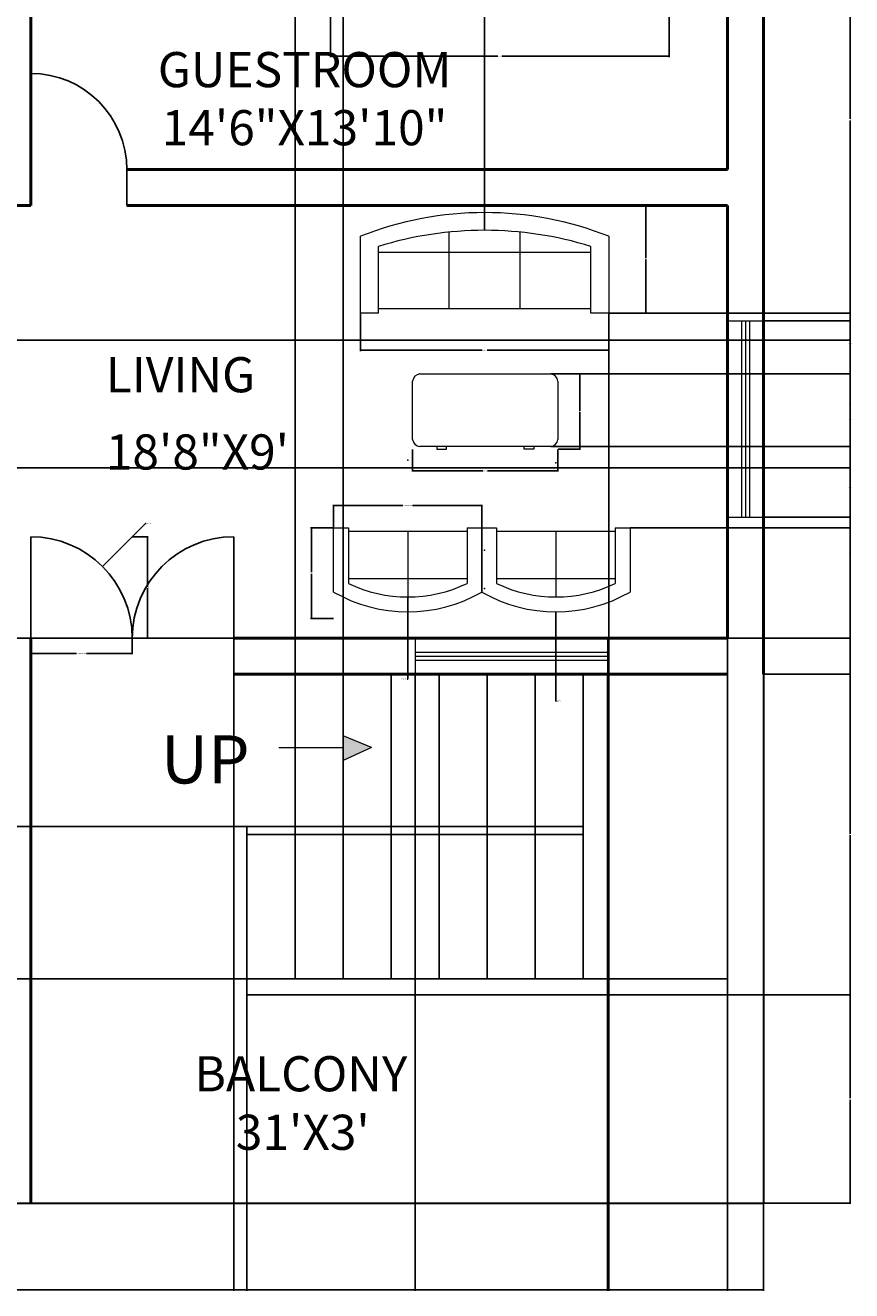
# Model space of a CAD drawing. Units: feet. Extents: x 2387 to 2818, y 1569 to 2046.
# Tile 3 of 4: x 2611 to 2818, y 1569 to 1885. Entities that reach past the tile are written whole.
import ezdxf

# ---------------------------------------------------------------- set-up
doc = ezdxf.new("R2010")
doc.units = ezdxf.units.FT
for name, color, linetype, lineweight in [('A-ANNO-DIMS', 2, 'Continuous', 18), ('A-ANNO-SYMB', 7, 'Continuous', 18), ('A-ANNO-TEXT', 7, 'Continuous', 18), ('A-AREA-IDEN', 7, 'Continuous', 18), ('A-DOOR', 3, 'Continuous', 25), ('A-FLOR-BALC', 7, 'Continuous', 30), ('A-FLOR-STRS', 7, 'Continuous', 25), ('A-FURN', 8, 'Continuous', 18), ('A-GLAZ', 4, 'Continuous', 18), ('A-WALL', 7, 'Continuous', 50)]:
    doc.layers.add(name, color=color, linetype=linetype, lineweight=lineweight)
doc.styles.get("Standard").update_dxf_attribs({"font": 'arial.ttf'})
doc.dimstyles.get("Standard").update_dxf_attribs({"dimtxt": 0.18, "dimasz": 0.18, "dimexe": 0.18, "dimexo": 0.0625, "dimgap": 0.09, "dimtad": 0, "dimtih": 1, "dimtoh": 1, "dimdec": 4, "dimzin": 0, "dimdsep": 46, "dimtxsty": 'Standard', "dimcen": 0.09, "dimadec": 0, "dimazin": 0, "dimtfac": 1, "dimtdec": 4, "dimtofl": 0, "dimtmove": 0, "dimatfit": 3, "dimfxl": 1, "dimtolj": 1, "dimtzin": 0, "dimarcsym": 0})

# ---------------------------------------------------------------- blocks, each defined once
blk = doc.blocks.new('Sofa - Roundback 7 ft.')
for p, q in [((-12.00002, -32.4421), (-12.00003, -6.5971)), ((11.99997, -32.4421), (11.99998, -6.5971)), ((-36.000027, -34), (-36.000027, -11.4696)), ((35.99998, -34), (35.99998, -11.4696)), ((-35.999844, -13.3819), (35.9998, -13.3819)), ((-36.000027, -32.4421), (35.99998, -32.4421))]:
    blk.add_line(p, q)
for points in [[(-36.000027, -34), (-42.000027, -34), (-42.000027, -8)], [(41.99998, -8), (41.99998, -34), (35.99998, -34)]]:
    blk.add_lwpolyline(points)
for centre, radius, start, end in [((0, -114.25), 114.25, 68.43141, 111.5686), ((-0.00001, -127.1968), 121.1968, 72.72033, 107.2797)]:
    blk.add_arc(centre, radius, start, end)
blk = doc.blocks.new('Desk - 30 x 60 in.')
for p, q in [((-26.999995, 0), (26.999995, 0)), ((-29.999995, -27), (-29.999995, -3)), ((29.999995, -3), (29.999995, -27)), ((26.999995, -30), (-26.999995, -30)), ((-20.000005, -30), (-20.000005, -31)), ((-20.000005, -31), (-16.000005, -31)), ((-16.000005, -31), (-16.000005, -30)), ((15.999995, -31), (15.999995, -30)), ((19.999995, -31), (15.999995, -31)), ((19.999995, -30), (19.999995, -31))]:
    blk.add_line(p, q)
for centre, start, end in [((-26.499995, -3.5), 98.1301, 171.8699), ((26.499995, -3.5), 8.130102, 81.8699), ((-26.499995, -26.5), 188.1301, 261.8699), ((26.499995, -26.5), 278.1301, 351.8699)]:
    blk.add_arc(centre, 3.535534, start, end)
blk = doc.blocks.new('Sofa - Roundback Loveseat 5 ft.')
for p, q in [((0, -32.44198), (0, -5.99998)), ((-24, -33.99998), (-24, -11.46958)), ((-23.9998, -13.38178), (23.99986, -13.38178)), ((24.00004, -33.99998), (24.00004, -11.46958)), ((-24, -32.44198), (24.00004, -32.44198))]:
    blk.add_line(p, q)
for points in [[(-24, -33.99998), (-30, -33.99998), (-30, -7.99998)], [(30.00004, -7.99998), (30.00004, -33.99998), (24.00004, -33.99998)]]:
    blk.add_lwpolyline(points)
for centre, radius, start, end in [((0, -60.24998), 60.24998, 60.13715, 119.8628), ((0, -61.38438), 55.38444, 64.32083, 115.6792)]:
    blk.add_arc(centre, radius, start, end)
blk = doc.blocks.new('DOOR-PAIRED-LEAF')
blk.add_line((0, 0), (0, 25.34))
blk.add_arc((0, 0), 25.34, 0, 90)
blk = doc.blocks.new('DOOR-BEDROOM-SWING')
blk.add_line((0, 9), (0, 0))
blk.add_arc((24, 9), 24, 90, 180)
blk = doc.blocks.new('*D12')
at = {"layer": 'A-ANNO-DIMS', "color": 0, "lineweight": -2, "transparency": 16777216}
for p, q in [((2687.62, 1893.93), (2687.62, 1876.9)), ((2772.16, 1893.93), (2772.16, 1876.9)), ((2687.8, 1877.08), (2729.36, 1877.08)), ((2771.98, 1877.08), (2730.42, 1877.08))]:
    blk.add_line(p, q, dxfattribs=at)
at = {"layer": 'A-ANNO-DIMS', "color": 0, "transparency": 16777216}
for points in [[(2687.8, 1877.11), (2687.8, 1877.05), (2687.62, 1877.08)], [(2771.98, 1877.11), (2771.98, 1877.05), (2772.16, 1877.08)]]:
    blk.add_solid(points, dxfattribs=at)
at = {"layer": 'Defpoints', "color": 0, "transparency": 16777216}
for p in [(2687.62, 1893.99), (2772.16, 1893.99), (2772.16, 1877.08)]:
    blk.add_point(p, dxfattribs=at)
at = {"layer": 'A-ANNO-DIMS', "color": 0, "transparency": 16777216, "insert": (2729.89, 1877.08), "char_height": 0.18, "attachment_point": 5}
blk.add_mtext('\\A1;85 TYP.', dxfattribs=at)
blk = doc.blocks.new('*D13')
at = {"layer": 'A-ANNO-DIMS', "color": 0, "lineweight": -2, "transparency": 16777216}
for p, q in [((2688.38, 1759.47), (2688.38, 1765.14)), ((2688.56, 1764.96), (2705.67, 1764.96)), ((2725.22, 1764.96), (2708.11, 1764.96)), ((2725.4, 1759.47), (2725.4, 1765.14))]:
    blk.add_line(p, q, dxfattribs=at)
at = {"layer": 'A-ANNO-DIMS', "color": 0, "transparency": 16777216}
for points in [[(2688.56, 1764.99), (2688.56, 1764.93), (2688.38, 1764.96)], [(2725.22, 1764.99), (2725.22, 1764.93), (2725.4, 1764.96)]]:
    blk.add_solid(points, dxfattribs=at)
at = {"layer": 'Defpoints', "color": 0, "transparency": 16777216}
for p in [(2688.38, 1764.96), (2688.38, 1759.41), (2725.4, 1759.41)]:
    blk.add_point(p, dxfattribs=at)
at = {"layer": 'A-ANNO-DIMS', "color": 0, "transparency": 16777216, "insert": (2706.89, 1764.96), "char_height": 0.18, "attachment_point": 5}
blk.add_mtext('\\A1;LOVESEAT 37 TYP.', dxfattribs=at)
blk = doc.blocks.new('*D14')
at = {"layer": 'A-ANNO-DIMS', "color": 0, "lineweight": -2, "transparency": 16777216}
for p, q in [((2688.31, 1759.41), (2682.64, 1759.41)), ((2682.82, 1759.23), (2682.82, 1748.28)), ((2682.82, 1736.96), (2682.82, 1747.91)), ((2688.31, 1736.78), (2682.64, 1736.78))]:
    blk.add_line(p, q, dxfattribs=at)
at = {"layer": 'A-ANNO-DIMS', "color": 0, "transparency": 16777216}
for points in [[(2682.79, 1759.23), (2682.85, 1759.23), (2682.82, 1759.41)], [(2682.79, 1736.96), (2682.85, 1736.96), (2682.82, 1736.78)]]:
    blk.add_solid(points, dxfattribs=at)
at = {"layer": 'Defpoints', "color": 0, "transparency": 16777216}
for p in [(2688.38, 1759.41), (2682.82, 1736.78), (2688.38, 1736.78)]:
    blk.add_point(p, dxfattribs=at)
at = {"layer": 'A-ANNO-DIMS', "color": 0, "transparency": 16777216, "insert": (2682.82, 1748.09), "char_height": 0.18, "attachment_point": 5}
blk.add_mtext('\\A1;23 TYP.', dxfattribs=at)
blk = doc.blocks.new('*D15')
at = {"layer": 'A-ANNO-DIMS', "color": 0, "lineweight": -2, "transparency": 16777216}
for p, q in [((2612.74, 1731.76), (2612.74, 1727.84)), ((2638.08, 1731.76), (2638.08, 1727.84)), ((2612.92, 1728.02), (2624.12, 1728.02)), ((2637.9, 1728.02), (2626.69, 1728.02))]:
    blk.add_line(p, q, dxfattribs=at)
at = {"layer": 'A-ANNO-DIMS', "color": 0, "transparency": 16777216}
for points in [[(2612.92, 1728.05), (2612.92, 1727.99), (2612.74, 1728.02)], [(2637.9, 1728.05), (2637.9, 1727.99), (2638.08, 1728.02)]]:
    blk.add_solid(points, dxfattribs=at)
at = {"layer": 'Defpoints', "color": 0, "transparency": 16777216}
for p in [(2612.74, 1731.82), (2638.08, 1731.82), (2638.08, 1728.02)]:
    blk.add_point(p, dxfattribs=at)
at = {"layer": 'A-ANNO-DIMS', "color": 0, "transparency": 16777216, "insert": (2625.41, 1728.02), "char_height": 0.18, "attachment_point": 5}
blk.add_mtext('\\A1;DOOR LEAF 25 TYP.', dxfattribs=at)
blk = doc.blocks.new('*D16')
at = {"layer": 'A-ANNO-DIMS', "color": 0, "lineweight": -2, "transparency": 16777216}
for p, q in [((2638.14, 1757.17), (2642.06, 1757.17)), ((2641.88, 1756.99), (2641.88, 1744.68)), ((2641.88, 1732), (2641.88, 1744.31)), ((2638.14, 1731.82), (2642.06, 1731.82))]:
    blk.add_line(p, q, dxfattribs=at)
at = {"layer": 'A-ANNO-DIMS', "color": 0, "transparency": 16777216}
for points in [[(2641.85, 1756.99), (2641.91, 1756.99), (2641.88, 1757.17)], [(2641.85, 1732), (2641.91, 1732), (2641.88, 1731.82)]]:
    blk.add_solid(points, dxfattribs=at)
at = {"layer": 'Defpoints', "color": 0, "transparency": 16777216}
for p in [(2638.08, 1757.17), (2641.88, 1757.17), (2638.08, 1731.82)]:
    blk.add_point(p, dxfattribs=at)
at = {"layer": 'A-ANNO-DIMS', "color": 0, "transparency": 16777216, "insert": (2641.88, 1744.5), "char_height": 0.18, "attachment_point": 5}
blk.add_mtext('\\A1;25 TYP.', dxfattribs=at)
blk = doc.blocks.new('*D21')
at = {"layer": 'A-ANNO-DIMS', "color": 0, "lineweight": -2, "transparency": 16777216}
for p, q in [((2695.12, 1812.93), (2695.12, 1803.52)), ((2757.09, 1812.93), (2757.09, 1803.52)), ((2695.3, 1803.7), (2725.51, 1803.7)), ((2756.91, 1803.7), (2726.7, 1803.7))]:
    blk.add_line(p, q, dxfattribs=at)
at = {"layer": 'A-ANNO-DIMS', "color": 0, "transparency": 16777216}
for points in [[(2695.3, 1803.73), (2695.3, 1803.67), (2695.12, 1803.7)], [(2756.91, 1803.73), (2756.91, 1803.67), (2757.09, 1803.7)]]:
    blk.add_solid(points, dxfattribs=at)
at = {"layer": 'Defpoints', "color": 0, "transparency": 16777216}
for p in [(2695.12, 1812.99), (2757.09, 1812.99), (2757.09, 1803.7)]:
    blk.add_point(p, dxfattribs=at)
at = {"layer": 'A-ANNO-DIMS', "color": 0, "transparency": 16777216, "insert": (2726.1, 1803.7), "char_height": 0.18, "attachment_point": 5}
blk.add_mtext('\\A1;SOFA 62', dxfattribs=at)
blk = doc.blocks.new('*D22')
at = {"layer": 'A-ANNO-DIMS', "color": 0, "lineweight": -2, "transparency": 16777216}
for p, q in [((2757.15, 1840.04), (2766.56, 1840.04)), ((2766.38, 1839.86), (2766.38, 1826.7)), ((2766.38, 1813.17), (2766.38, 1826.34)), ((2757.15, 1812.99), (2766.56, 1812.99))]:
    blk.add_line(p, q, dxfattribs=at)
at = {"layer": 'A-ANNO-DIMS', "color": 0, "transparency": 16777216}
for points in [[(2766.35, 1839.86), (2766.41, 1839.86), (2766.38, 1840.04)], [(2766.35, 1813.17), (2766.41, 1813.17), (2766.38, 1812.99)]]:
    blk.add_solid(points, dxfattribs=at)
at = {"layer": 'Defpoints', "color": 0, "transparency": 16777216}
for p in [(2757.09, 1840.04), (2766.38, 1840.04), (2757.09, 1812.99)]:
    blk.add_point(p, dxfattribs=at)
at = {"layer": 'A-ANNO-DIMS', "color": 0, "transparency": 16777216, "insert": (2766.38, 1826.52), "char_height": 0.18, "attachment_point": 5}
blk.add_mtext('\\A1;27', dxfattribs=at)
blk = doc.blocks.new('*D23')
at = {"layer": 'A-ANNO-DIMS', "color": 0, "lineweight": -2, "transparency": 16777216}
for p, q in [((2708.1, 1778.98), (2708.1, 1773.41)), ((2744.42, 1778.98), (2744.42, 1773.41)), ((2708.28, 1773.59), (2725.67, 1773.59)), ((2744.24, 1773.59), (2726.85, 1773.59))]:
    blk.add_line(p, q, dxfattribs=at)
at = {"layer": 'A-ANNO-DIMS', "color": 0, "transparency": 16777216}
for points in [[(2708.28, 1773.62), (2708.28, 1773.56), (2708.1, 1773.59)], [(2744.24, 1773.62), (2744.24, 1773.56), (2744.42, 1773.59)]]:
    blk.add_solid(points, dxfattribs=at)
at = {"layer": 'Defpoints', "color": 0, "transparency": 16777216}
for p in [(2708.1, 1779.04), (2744.42, 1779.04), (2744.42, 1773.59)]:
    blk.add_point(p, dxfattribs=at)
at = {"layer": 'A-ANNO-DIMS', "color": 0, "transparency": 16777216, "insert": (2726.26, 1773.59), "char_height": 0.18, "attachment_point": 5}
blk.add_mtext('\\A1;DESK 36', dxfattribs=at)
blk = doc.blocks.new('*D24')
at = {"layer": 'A-ANNO-DIMS', "color": 0, "lineweight": -2, "transparency": 16777216}
for p, q in [((2744.48, 1797.81), (2750.05, 1797.81)), ((2749.87, 1797.63), (2749.87, 1788.61)), ((2749.87, 1779.22), (2749.87, 1788.24)), ((2744.48, 1779.04), (2750.05, 1779.04))]:
    blk.add_line(p, q, dxfattribs=at)
at = {"layer": 'A-ANNO-DIMS', "color": 0, "transparency": 16777216}
for points in [[(2749.84, 1797.63), (2749.9, 1797.63), (2749.87, 1797.81)], [(2749.84, 1779.22), (2749.9, 1779.22), (2749.87, 1779.04)]]:
    blk.add_solid(points, dxfattribs=at)
at = {"layer": 'Defpoints', "color": 0, "transparency": 16777216}
for p in [(2744.42, 1797.81), (2749.87, 1797.81), (2744.42, 1779.04)]:
    blk.add_point(p, dxfattribs=at)
at = {"layer": 'A-ANNO-DIMS', "color": 0, "transparency": 16777216, "insert": (2749.87, 1788.43), "char_height": 0.18, "attachment_point": 5}
blk.add_mtext('\\A1;19', dxfattribs=at)
blk = doc.blocks.new('*D27')
at = {"layer": 'A-ANNO-DIMS', "color": 0, "lineweight": -2, "transparency": 16777216}
for p, q in [((2408.74, 1590.76), (2408.74, 1568.96)), ((2795.74, 1590.76), (2795.74, 1568.96)), ((2408.92, 1569.14), (2601.95, 1569.14)), ((2795.56, 1569.14), (2602.52, 1569.14))]:
    blk.add_line(p, q, dxfattribs=at)
at = {"layer": 'A-ANNO-DIMS', "color": 0, "transparency": 16777216}
for points in [[(2408.92, 1569.17), (2408.92, 1569.11), (2408.74, 1569.14)], [(2795.56, 1569.17), (2795.56, 1569.11), (2795.74, 1569.14)]]:
    blk.add_solid(points, dxfattribs=at)
at = {"layer": 'Defpoints', "color": 0, "transparency": 16777216}
for p in [(2408.74, 1590.82), (2795.74, 1590.82), (2795.74, 1569.14)]:
    blk.add_point(p, dxfattribs=at)
at = {"layer": 'A-ANNO-DIMS', "color": 0, "transparency": 16777216, "insert": (2602.24, 1569.14), "char_height": 0.18, "attachment_point": 5}
blk.add_mtext('\\A1;387', dxfattribs=at)
blk = doc.blocks.new('*D50')
at = {"layer": 'A-ANNO-DIMS', "color": 0, "lineweight": -2, "transparency": 16777216}
for p, q in [((2795.8, 1642.82), (2817.6, 1642.82)), ((2817.42, 1642.64), (2817.42, 1617.01)), ((2817.42, 1591), (2817.42, 1616.64)), ((2795.8, 1590.82), (2817.6, 1590.82))]:
    blk.add_line(p, q, dxfattribs=at)
at = {"layer": 'A-ANNO-DIMS', "color": 0, "transparency": 16777216}
for points in [[(2817.39, 1642.64), (2817.45, 1642.64), (2817.42, 1642.82)], [(2817.39, 1591), (2817.45, 1591), (2817.42, 1590.82)]]:
    blk.add_solid(points, dxfattribs=at)
at = {"layer": 'Defpoints', "color": 0, "transparency": 16777216}
for p in [(2795.74, 1642.82), (2817.42, 1642.82), (2795.74, 1590.82)]:
    blk.add_point(p, dxfattribs=at)
at = {"layer": 'A-ANNO-DIMS', "color": 0, "transparency": 16777216, "insert": (2817.42, 1616.82), "char_height": 0.18, "attachment_point": 5}
blk.add_mtext('\\A1;52', dxfattribs=at)
blk = doc.blocks.new('*D51')
at = {"layer": 'A-ANNO-DIMS', "color": 0, "lineweight": -2, "transparency": 16777216}
for p, q in [((2795.8, 1722.82), (2817.6, 1722.82)), ((2817.42, 1722.64), (2817.42, 1683.01)), ((2817.42, 1643), (2817.42, 1682.64)), ((2795.8, 1642.82), (2817.6, 1642.82))]:
    blk.add_line(p, q, dxfattribs=at)
at = {"layer": 'A-ANNO-DIMS', "color": 0, "transparency": 16777216}
for points in [[(2817.39, 1722.64), (2817.45, 1722.64), (2817.42, 1722.82)], [(2817.39, 1643), (2817.45, 1643), (2817.42, 1642.82)]]:
    blk.add_solid(points, dxfattribs=at)
at = {"layer": 'Defpoints', "color": 0, "transparency": 16777216}
for p in [(2795.74, 1722.82), (2817.42, 1722.82), (2795.74, 1642.82)]:
    blk.add_point(p, dxfattribs=at)
at = {"layer": 'A-ANNO-DIMS', "color": 0, "transparency": 16777216, "insert": (2817.42, 1682.82), "char_height": 0.18, "attachment_point": 5}
blk.add_mtext('\\A1;80', dxfattribs=at)
blk = doc.blocks.new('*D52')
at = {"layer": 'A-ANNO-DIMS', "color": 0, "lineweight": -2, "transparency": 16777216}
for p, q in [((2795.8, 1762.05), (2817.6, 1762.05)), ((2817.42, 1761.87), (2817.42, 1742.62)), ((2817.42, 1723), (2817.42, 1742.26)), ((2795.8, 1722.82), (2817.6, 1722.82))]:
    blk.add_line(p, q, dxfattribs=at)
at = {"layer": 'A-ANNO-DIMS', "color": 0, "transparency": 16777216}
for points in [[(2817.39, 1761.87), (2817.45, 1761.87), (2817.42, 1762.05)], [(2817.39, 1723), (2817.45, 1723), (2817.42, 1722.82)]]:
    blk.add_solid(points, dxfattribs=at)
at = {"layer": 'Defpoints', "color": 0, "transparency": 16777216}
for p in [(2795.74, 1762.05), (2817.42, 1762.05), (2795.74, 1722.82)]:
    blk.add_point(p, dxfattribs=at)
at = {"layer": 'A-ANNO-DIMS', "color": 0, "transparency": 16777216, "insert": (2817.42, 1742.44), "char_height": 0.18, "attachment_point": 5}
blk.add_mtext('\\A1;39.23', dxfattribs=at)
blk = doc.blocks.new('*D53')
at = {"layer": 'A-ANNO-DIMS', "color": 0, "lineweight": -2, "transparency": 16777216}
for p, q in [((2795.8, 1811.02), (2817.6, 1811.02)), ((2817.42, 1810.84), (2817.42, 1786.72)), ((2817.42, 1762.23), (2817.42, 1786.36)), ((2795.8, 1762.05), (2817.6, 1762.05))]:
    blk.add_line(p, q, dxfattribs=at)
at = {"layer": 'A-ANNO-DIMS', "color": 0, "transparency": 16777216}
for points in [[(2817.39, 1810.84), (2817.45, 1810.84), (2817.42, 1811.02)], [(2817.39, 1762.23), (2817.45, 1762.23), (2817.42, 1762.05)]]:
    blk.add_solid(points, dxfattribs=at)
at = {"layer": 'Defpoints', "color": 0, "transparency": 16777216}
for p in [(2795.74, 1811.02), (2817.42, 1811.02), (2795.74, 1762.05)]:
    blk.add_point(p, dxfattribs=at)
at = {"layer": 'A-ANNO-DIMS', "color": 0, "transparency": 16777216, "insert": (2817.42, 1786.54), "char_height": 0.18, "attachment_point": 5}
blk.add_mtext('\\A1;48.97', dxfattribs=at)
blk = doc.blocks.new('*D54')
at = {"layer": 'A-ANNO-DIMS', "color": 0, "lineweight": -2, "transparency": 16777216}
for p, q in [((2795.8, 1911.52), (2817.6, 1911.52)), ((2817.42, 1911.34), (2817.42, 1861.45)), ((2817.42, 1811.2), (2817.42, 1861.09)), ((2795.8, 1811.02), (2817.6, 1811.02))]:
    blk.add_line(p, q, dxfattribs=at)
at = {"layer": 'A-ANNO-DIMS', "color": 0, "transparency": 16777216}
for points in [[(2817.39, 1911.34), (2817.45, 1911.34), (2817.42, 1911.52)], [(2817.39, 1811.2), (2817.45, 1811.2), (2817.42, 1811.02)]]:
    blk.add_solid(points, dxfattribs=at)
at = {"layer": 'Defpoints', "color": 0, "transparency": 16777216}
for p in [(2795.74, 1911.52), (2817.42, 1911.52), (2795.74, 1811.02)]:
    blk.add_point(p, dxfattribs=at)
at = {"layer": 'A-ANNO-DIMS', "color": 0, "transparency": 16777216, "insert": (2817.42, 1861.27), "char_height": 0.18, "attachment_point": 5}
blk.add_mtext('\\A1;100.5', dxfattribs=at)
blk = doc.blocks.new('*D57')
at = {"layer": 'A-ANNO-DIMS', "color": 0, "lineweight": -2, "transparency": 16777216}
for p, q in [((2666.74, 1642.76), (2666.74, 1568.96)), ((2795.74, 1642.76), (2795.74, 1568.96)), ((2666.92, 1569.14), (2730.96, 1569.14)), ((2795.56, 1569.14), (2731.52, 1569.14))]:
    blk.add_line(p, q, dxfattribs=at)
at = {"layer": 'A-ANNO-DIMS', "color": 0, "transparency": 16777216}
for points in [[(2666.92, 1569.17), (2666.92, 1569.11), (2666.74, 1569.14)], [(2795.56, 1569.17), (2795.56, 1569.11), (2795.74, 1569.14)]]:
    blk.add_solid(points, dxfattribs=at)
at = {"layer": 'Defpoints', "color": 0, "transparency": 16777216}
for p in [(2666.74, 1642.82), (2795.74, 1642.82), (2795.74, 1569.14)]:
    blk.add_point(p, dxfattribs=at)
at = {"layer": 'A-ANNO-DIMS', "color": 0, "transparency": 16777216, "insert": (2731.24, 1569.14), "char_height": 0.18, "attachment_point": 5}
blk.add_mtext('\\A1;129', dxfattribs=at)
blk = doc.blocks.new('*D58')
at = {"layer": 'A-ANNO-DIMS', "color": 0, "lineweight": -2, "transparency": 16777216}
for p, q in [((2678.74, 1646.89), (2678.74, 2045.68)), ((2678.92, 2045.5), (2684.53, 2045.5)), ((2690.56, 2045.5), (2684.95, 2045.5)), ((2690.74, 1646.89), (2690.74, 2045.68))]:
    blk.add_line(p, q, dxfattribs=at)
at = {"layer": 'A-ANNO-DIMS', "color": 0, "transparency": 16777216}
for points in [[(2678.92, 2045.53), (2678.92, 2045.47), (2678.74, 2045.5)], [(2690.56, 2045.53), (2690.56, 2045.47), (2690.74, 2045.5)]]:
    blk.add_solid(points, dxfattribs=at)
at = {"layer": 'Defpoints', "color": 0, "transparency": 16777216}
for p in [(2690.74, 2045.5), (2678.74, 1646.82), (2690.74, 1646.82)]:
    blk.add_point(p, dxfattribs=at)
at = {"layer": 'A-ANNO-DIMS', "color": 0, "transparency": 16777216, "insert": (2684.74, 2045.5), "char_height": 0.18, "attachment_point": 5}
blk.add_mtext('\\A1;12', dxfattribs=at)
blk = doc.blocks.new('*D59')
at = {"layer": 'A-ANNO-DIMS', "color": 0, "lineweight": -2, "transparency": 16777216}
for p, q in [((2666.67, 1684.82), (2386.88, 1684.82)), ((2387.06, 1684.64), (2387.06, 1666.01)), ((2387.06, 1647), (2387.06, 1665.64)), ((2666.67, 1646.82), (2386.88, 1646.82))]:
    blk.add_line(p, q, dxfattribs=at)
at = {"layer": 'A-ANNO-DIMS', "color": 0, "transparency": 16777216}
for points in [[(2387.03, 1684.64), (2387.09, 1684.64), (2387.06, 1684.82)], [(2387.03, 1647), (2387.09, 1647), (2387.06, 1646.82)]]:
    blk.add_solid(points, dxfattribs=at)
at = {"layer": 'Defpoints', "color": 0, "transparency": 16777216}
for p in [(2666.74, 1684.82), (2387.06, 1646.82), (2666.74, 1646.82)]:
    blk.add_point(p, dxfattribs=at)
at = {"layer": 'A-ANNO-DIMS', "color": 0, "transparency": 16777216, "insert": (2387.06, 1665.82), "char_height": 0.18, "attachment_point": 5}
blk.add_mtext('\\A1;38', dxfattribs=at)
blk = doc.blocks.new('*D60')
at = {"layer": 'A-ANNO-DIMS', "color": 0, "lineweight": -2, "transparency": 16777216}
for p, q in [((2663.42, 1722.76), (2663.42, 1568.96)), ((2708.76, 1722.76), (2708.76, 1568.96)), ((2663.6, 1569.14), (2685.7, 1569.14)), ((2708.58, 1569.14), (2686.49, 1569.14))]:
    blk.add_line(p, q, dxfattribs=at)
at = {"layer": 'A-ANNO-DIMS', "color": 0, "transparency": 16777216}
for points in [[(2663.6, 1569.17), (2663.6, 1569.11), (2663.42, 1569.14)], [(2708.58, 1569.17), (2708.58, 1569.11), (2708.76, 1569.14)]]:
    blk.add_solid(points, dxfattribs=at)
at = {"layer": 'Defpoints', "color": 0, "transparency": 16777216}
for p in [(2663.42, 1722.82), (2708.76, 1722.82), (2708.76, 1569.14)]:
    blk.add_point(p, dxfattribs=at)
at = {"layer": 'A-ANNO-DIMS', "color": 0, "transparency": 16777216, "insert": (2686.09, 1569.14), "char_height": 0.18, "attachment_point": 5}
blk.add_mtext('\\A1;45.34', dxfattribs=at)
blk = doc.blocks.new('*D61')
at = {"layer": 'A-ANNO-DIMS', "color": 0, "lineweight": -2, "transparency": 16777216}
for p, q in [((2708.76, 1722.76), (2708.76, 1568.96)), ((2756.83, 1722.76), (2756.83, 1568.96)), ((2708.94, 1569.14), (2732.4, 1569.14)), ((2756.65, 1569.14), (2733.19, 1569.14))]:
    blk.add_line(p, q, dxfattribs=at)
at = {"layer": 'A-ANNO-DIMS', "color": 0, "transparency": 16777216}
for points in [[(2708.94, 1569.17), (2708.94, 1569.11), (2708.76, 1569.14)], [(2756.65, 1569.17), (2756.65, 1569.11), (2756.83, 1569.14)]]:
    blk.add_solid(points, dxfattribs=at)
at = {"layer": 'Defpoints', "color": 0, "transparency": 16777216}
for p in [(2708.76, 1722.82), (2756.83, 1722.82), (2756.83, 1569.14)]:
    blk.add_point(p, dxfattribs=at)
at = {"layer": 'A-ANNO-DIMS', "color": 0, "transparency": 16777216, "insert": (2732.8, 1569.14), "char_height": 0.18, "attachment_point": 5}
blk.add_mtext('\\A1;48.06', dxfattribs=at)
blk = doc.blocks.new('*D62')
at = {"layer": 'A-ANNO-DIMS', "color": 0, "lineweight": -2, "transparency": 16777216}
for p, q in [((2567.8, 1806.26), (2817.6, 1806.26)), ((2817.42, 1806.08), (2817.42, 1790.49)), ((2817.42, 1774.54), (2817.42, 1790.13)), ((2567.8, 1774.36), (2817.6, 1774.36))]:
    blk.add_line(p, q, dxfattribs=at)
at = {"layer": 'A-ANNO-DIMS', "color": 0, "transparency": 16777216}
for points in [[(2817.39, 1806.08), (2817.45, 1806.08), (2817.42, 1806.26)], [(2817.39, 1774.54), (2817.45, 1774.54), (2817.42, 1774.36)]]:
    blk.add_solid(points, dxfattribs=at)
at = {"layer": 'Defpoints', "color": 0, "transparency": 16777216}
for p in [(2567.74, 1806.26), (2817.42, 1806.26), (2567.74, 1774.36)]:
    blk.add_point(p, dxfattribs=at)
at = {"layer": 'A-ANNO-DIMS', "color": 0, "transparency": 16777216, "insert": (2817.42, 1790.31), "char_height": 0.18, "attachment_point": 5}
blk.add_mtext('\\A1;31.904', dxfattribs=at)
blk = doc.blocks.new('*D63')
at = {"layer": 'A-ANNO-DIMS', "color": 0, "lineweight": -2, "transparency": 16777216}
for p, q in [((2567.8, 1774.36), (2817.6, 1774.36)), ((2817.42, 1774.18), (2817.42, 1753.27)), ((2817.42, 1732), (2817.42, 1752.91)), ((2567.8, 1731.82), (2817.6, 1731.82))]:
    blk.add_line(p, q, dxfattribs=at)
at = {"layer": 'A-ANNO-DIMS', "color": 0, "transparency": 16777216}
for points in [[(2817.39, 1774.18), (2817.45, 1774.18), (2817.42, 1774.36)], [(2817.39, 1732), (2817.45, 1732), (2817.42, 1731.82)]]:
    blk.add_solid(points, dxfattribs=at)
at = {"layer": 'Defpoints', "color": 0, "transparency": 16777216}
for p in [(2567.74, 1774.36), (2817.42, 1774.36), (2567.74, 1731.82)]:
    blk.add_point(p, dxfattribs=at)
at = {"layer": 'A-ANNO-DIMS', "color": 0, "transparency": 16777216, "insert": (2817.42, 1753.09), "char_height": 0.18, "attachment_point": 5}
blk.add_mtext('\\A1;42.53', dxfattribs=at)
blk = doc.blocks.new('*D69')
at = {"layer": 'A-ANNO-DIMS', "color": 0, "lineweight": -2, "transparency": 16777216}
for p, q in [((2757.09, 1812.93), (2757.09, 1568.96)), ((2786.74, 1810.96), (2786.74, 1568.96)), ((2757.27, 1569.14), (2771.51, 1569.14)), ((2786.56, 1569.14), (2772.31, 1569.14))]:
    blk.add_line(p, q, dxfattribs=at)
at = {"layer": 'A-ANNO-DIMS', "color": 0, "transparency": 16777216}
for points in [[(2757.27, 1569.17), (2757.27, 1569.11), (2757.09, 1569.14)], [(2786.56, 1569.17), (2786.56, 1569.11), (2786.74, 1569.14)]]:
    blk.add_solid(points, dxfattribs=at)
at = {"layer": 'Defpoints', "color": 0, "transparency": 16777216}
for p in [(2757.09, 1812.99), (2786.74, 1811.02), (2786.74, 1569.14)]:
    blk.add_point(p, dxfattribs=at)
at = {"layer": 'A-ANNO-DIMS', "color": 0, "transparency": 16777216, "insert": (2771.91, 1569.14), "char_height": 0.18, "attachment_point": 5}
blk.add_mtext('\\A1;29.65', dxfattribs=at)
blk = doc.blocks.new('*D70')
at = {"layer": 'A-ANNO-DIMS', "color": 0, "lineweight": -2, "transparency": 16777216}
for p, q in [((2757.15, 1812.99), (2817.6, 1812.99)), ((2817.42, 1812.81), (2817.42, 1805.58)), ((2817.42, 1797.99), (2817.42, 1805.22)), ((2742.67, 1797.81), (2817.6, 1797.81))]:
    blk.add_line(p, q, dxfattribs=at)
at = {"layer": 'A-ANNO-DIMS', "color": 0, "transparency": 16777216}
for points in [[(2817.39, 1812.81), (2817.45, 1812.81), (2817.42, 1812.99)], [(2817.39, 1797.99), (2817.45, 1797.99), (2817.42, 1797.81)]]:
    blk.add_solid(points, dxfattribs=at)
at = {"layer": 'Defpoints', "color": 0, "transparency": 16777216}
for p in [(2757.09, 1812.99), (2742.6, 1797.81), (2817.42, 1797.81)]:
    blk.add_point(p, dxfattribs=at)
at = {"layer": 'A-ANNO-DIMS', "color": 0, "transparency": 16777216, "insert": (2817.42, 1805.4), "char_height": 0.18, "attachment_point": 5}
blk.add_mtext('\\A1;15.185', dxfattribs=at)
blk = doc.blocks.new('*D71')
at = {"layer": 'A-ANNO-DIMS', "color": 0, "lineweight": -2, "transparency": 16777216}
for p, q in [((2742.67, 1779.65), (2817.6, 1779.65)), ((2817.42, 1779.47), (2817.42, 1769.71)), ((2817.42, 1759.59), (2817.42, 1769.35)), ((2762.49, 1759.41), (2817.6, 1759.41))]:
    blk.add_line(p, q, dxfattribs=at)
at = {"layer": 'A-ANNO-DIMS', "color": 0, "transparency": 16777216}
for points in [[(2817.39, 1779.47), (2817.45, 1779.47), (2817.42, 1779.65)], [(2817.39, 1759.59), (2817.45, 1759.59), (2817.42, 1759.41)]]:
    blk.add_solid(points, dxfattribs=at)
at = {"layer": 'Defpoints', "color": 0, "transparency": 16777216}
for p in [(2742.6, 1779.65), (2817.42, 1779.65), (2762.42, 1759.41)]:
    blk.add_point(p, dxfattribs=at)
at = {"layer": 'A-ANNO-DIMS', "color": 0, "transparency": 16777216, "insert": (2817.42, 1769.53), "char_height": 0.18, "attachment_point": 5}
blk.add_mtext('\\A1;20.242', dxfattribs=at)
blk = doc.blocks.new('*D74')
at = {"layer": 'A-ANNO-DIMS', "color": 0, "lineweight": -2, "transparency": 16777216}
for p, q in [((2641.41, 1760.5), (2630.78, 1749.87)), ((2641.59, 1760.5), (2641.41, 1760.5)), ((2612.65, 1731.82), (2612.83, 1731.82)), ((2612.74, 1731.73), (2612.74, 1731.91))]:
    blk.add_line(p, q, dxfattribs=at)
at = {"layer": 'A-ANNO-DIMS', "color": 0, "transparency": 16777216}
blk.add_solid([(2630.76, 1749.89), (2630.8, 1749.85), (2630.66, 1749.74)], dxfattribs=at)
at = {"layer": 'Defpoints', "color": 0, "transparency": 16777216}
for p in [(2630.66, 1749.74), (2612.74, 1731.82)]:
    blk.add_point(p, dxfattribs=at)
at = {"layer": 'A-ANNO-DIMS', "color": 0, "transparency": 16777216, "insert": (2642.33, 1760.5), "char_height": 0.18, "attachment_point": 5}
blk.add_mtext('\\A1;2X R25.343', dxfattribs=at)
blk = doc.blocks.new('*D76')
at = {"layer": 'A-ANNO-DIMS', "color": 0, "lineweight": -2, "transparency": 16777216}
for p, q in [((2726.29, 1887.29), (2726.1, 1887.29)), ((2726.1, 1887.29), (2726.1, 1833.83)), ((2726.01, 1744.25), (2726.19, 1744.25)), ((2726.1, 1744.16), (2726.1, 1744.34))]:
    blk.add_line(p, q, dxfattribs=at)
at = {"layer": 'A-ANNO-DIMS', "color": 0, "transparency": 16777216}
blk.add_solid([(2726.08, 1833.83), (2726.14, 1833.83), (2726.1, 1833.65)], dxfattribs=at)
at = {"layer": 'Defpoints', "color": 0, "transparency": 16777216}
for p in [(2726.1, 1833.65), (2726.1, 1744.25)]:
    blk.add_point(p, dxfattribs=at)
at = {"layer": 'A-ANNO-DIMS', "color": 0, "transparency": 16777216, "insert": (2726.69, 1887.29), "char_height": 0.18, "attachment_point": 5}
blk.add_mtext('\\A1;R89.4', dxfattribs=at)
blk = doc.blocks.new('*D77')
at = {"layer": 'A-ANNO-DIMS', "color": 0, "lineweight": -2, "transparency": 16777216}
for p, q in [((2726.29, 1888.64), (2726.1, 1888.64)), ((2726.1, 1888.64), (2726.1, 1838.25)), ((2726.01, 1753.8), (2726.19, 1753.8)), ((2726.1, 1753.71), (2726.1, 1753.89))]:
    blk.add_line(p, q, dxfattribs=at)
at = {"layer": 'A-ANNO-DIMS', "color": 0, "transparency": 16777216}
blk.add_solid([(2726.08, 1838.25), (2726.14, 1838.25), (2726.1, 1838.07)], dxfattribs=at)
at = {"layer": 'Defpoints', "color": 0, "transparency": 16777216}
for p in [(2726.1, 1838.07), (2726.1, 1753.8)]:
    blk.add_point(p, dxfattribs=at)
at = {"layer": 'A-ANNO-DIMS', "color": 0, "transparency": 16777216, "insert": (2726.76, 1888.64), "char_height": 0.18, "attachment_point": 5}
blk.add_mtext('\\A1;R84.27', dxfattribs=at)
blk = doc.blocks.new('*D78')
at = {"layer": 'A-ANNO-DIMS', "color": 0, "lineweight": -2, "transparency": 16777216}
for p, q in [((2743.82, 1775.6), (2744, 1775.6)), ((2743.91, 1775.51), (2743.91, 1775.69)), ((2743.91, 1716.12), (2743.91, 1738.25)), ((2744.09, 1716.12), (2743.91, 1716.12))]:
    blk.add_line(p, q, dxfattribs=at)
at = {"layer": 'A-ANNO-DIMS', "color": 0, "transparency": 16777216}
blk.add_solid([(2743.94, 1738.25), (2743.88, 1738.25), (2743.91, 1738.43)], dxfattribs=at)
at = {"layer": 'Defpoints', "color": 0, "transparency": 16777216}
for p in [(2743.91, 1775.6), (2743.91, 1738.43)]:
    blk.add_point(p, dxfattribs=at)
at = {"layer": 'A-ANNO-DIMS', "color": 0, "transparency": 16777216, "insert": (2744.77, 1716.12), "char_height": 0.18, "attachment_point": 5}
blk.add_mtext('\\A1;2X R37.18', dxfattribs=at)
blk = doc.blocks.new('*D79')
at = {"layer": 'A-ANNO-DIMS', "color": 0, "lineweight": -2, "transparency": 16777216}
for p, q in [((2706.8, 1776.3), (2706.98, 1776.3)), ((2706.89, 1776.21), (2706.89, 1776.39)), ((2706.89, 1721.62), (2706.89, 1741.95)), ((2706.71, 1721.62), (2706.89, 1721.62))]:
    blk.add_line(p, q, dxfattribs=at)
at = {"layer": 'A-ANNO-DIMS', "color": 0, "transparency": 16777216}
blk.add_solid([(2706.86, 1741.95), (2706.92, 1741.95), (2706.89, 1742.13)], dxfattribs=at)
at = {"layer": 'Defpoints', "color": 0, "transparency": 16777216}
for p in [(2706.89, 1776.3), (2706.89, 1742.13)]:
    blk.add_point(p, dxfattribs=at)
at = {"layer": 'A-ANNO-DIMS', "color": 0, "transparency": 16777216, "insert": (2705.96, 1721.62), "char_height": 0.18, "attachment_point": 5}
blk.add_mtext('\\A1;2X R34.175', dxfattribs=at)

msp = doc.modelspace()

# ---------------------------------------------------------------- hatches: boundary and pattern name
at = {"layer": 'A-ANNO-SYMB'}
h = msp.add_hatch(color=256, dxfattribs=at)
h.dxf.hatch_style = 1
h.paths.add_polyline_path([(2690.736, 1707.4853), (2690.736, 1701.3138), (2697.8096, 1704.5875)])

# ---------------------------------------------------------------- linework, layer by layer
for p, q in [((2697.8096, 1704.5875), (2690.736, 1707.4853)), ((2674.6658, 1704.5875), (2690.736, 1704.5875)), ((2697.8096, 1704.5875), (2690.736, 1701.3138))]:
    msp.add_line(p, q, dxfattribs=at)
at = {"layer": 'A-DOOR'}
for p, q in [((2612.736, 1731.8244), (2603.736, 1731.8244)), ((2663.4216, 1731.8244), (2663.4216, 1722.8244))]:
    msp.add_line(p, q, dxfattribs=at)
at = {"layer": 'A-FLOR-BALC'}
for p in [(2795.736, 1722.8244), (2408.736, 1590.8244)]:
    msp.add_line(p, (2795.736, 1590.8244), dxfattribs=at)
at = {"layer": 'A-FLOR-STRS'}
for p, q in [((2678.736, 1722.8244), (2678.736, 1646.8244)), ((2690.736, 1722.8244), (2690.736, 1646.8244)), ((2702.736, 1722.8244), (2702.736, 1646.8244)), ((2714.736, 1722.8244), (2714.736, 1646.8244)), ((2726.736, 1722.8244), (2726.736, 1646.8244)), ((2738.736, 1722.8244), (2738.736, 1646.8244)), ((2750.736, 1722.8244), (2750.736, 1646.8244)), ((2786.736, 1722.8244), (2786.736, 1646.8244)), ((2786.736, 1722.8244), (2786.736, 1646.8244)), ((2750.736, 1684.8244), (2666.736, 1684.8244)), ((2666.736, 1684.8244), (2666.736, 1642.8244)), ((2750.736, 1682.8244), (2666.736, 1682.8244)), ((2786.736, 1646.8244), (2666.736, 1646.8244)), ((2795.736, 1642.8244), (2666.736, 1642.8244))]:
    msp.add_line(p, q, dxfattribs=at)
at = {"layer": 'A-GLAZ'}
for p, q in [((2786.736, 1811.0226), (2795.736, 1811.0226)), ((2790.236, 1811.0226), (2790.236, 1762.0537)), ((2791.236, 1811.0226), (2791.236, 1762.0537)), ((2792.236, 1811.0226), (2792.236, 1762.0537)), ((2786.736, 1762.0537), (2795.736, 1762.0537)), ((2708.7637, 1731.8244), (2708.7637, 1722.8244)), ((2756.8277, 1731.8244), (2756.8277, 1722.8244)), ((2708.7637, 1728.3244), (2756.8277, 1728.3244)), ((2708.7637, 1727.3244), (2756.8277, 1727.3244)), ((2708.7637, 1726.3244), (2756.8277, 1726.3244))]:
    msp.add_line(p, q, dxfattribs=at)
at = {"layer": 'A-WALL'}
for p, q in [((2795.736, 2023.8244), (2795.736, 1722.8244)), ((2612.736, 2014.8244), (2612.736, 1839.8244)), ((2786.736, 2014.8244), (2786.736, 1848.8244)), ((2786.736, 1848.8244), (2636.736, 1848.8244)), ((2612.736, 1839.8244), (2603.736, 1839.8244)), ((2786.736, 1839.8244), (2636.736, 1839.8244)), ((2786.736, 1839.8244), (2636.736, 1839.8244)), ((2786.736, 1839.8244), (2786.736, 1731.8244)), ((2795.736, 1839.8244), (2795.736, 1722.8244)), ((2612.736, 1590.8244), (2612.736, 1731.8244)), ((2786.736, 1731.8244), (2663.4216, 1731.8244)), ((2725.0788, 1731.8244), (2758.1037, 1731.8244)), ((2786.736, 1722.8244), (2663.4216, 1722.8244))]:
    msp.add_line(p, q, dxfattribs=at)

# ---------------------------------------------------------------- block references
at = {"layer": 'A-DOOR', "extrusion": (0, 0, -1), "zscale": -1}
for name, p in [('DOOR-BEDROOM-SWING', (-2636.7359, 1839.824)), ('DOOR-PAIRED-LEAF', (-2663.4216, 1731.824))]:
    msp.add_blockref(name, p, dxfattribs=at)
at = {"layer": 'A-DOOR'}
msp.add_blockref('DOOR-PAIRED-LEAF', (2612.736, 1731.824), dxfattribs=at)
at = {"layer": 'A-FURN'}
for name, p, xscale, yscale, zscale in [('Sofa - Roundback 7 ft.', (2726.1049, 1838.0742), 0.7376316609578243, 0.7376316609578243, 0.7376316609578243), ('Desk - 30 x 60 in.', (2726.2595, 1797.8097), 0.6053793579721252, 0.6053793579721252, 0.6053793579721252)]:
    msp.add_blockref(name, p, dxfattribs=dict(at, xscale=xscale, yscale=yscale, zscale=zscale))
at = {"layer": 'A-FURN', "xscale": 0.617058249960121, "yscale": 0.617058249960121, "zscale": 0.617058249960121, "rotation": 180}
for p in [(2706.8891, 1738.4263), (2743.9126, 1738.4263)]:
    msp.add_blockref('Sofa - Roundback Loveseat 5 ft.', p, dxfattribs=at)

# ---------------------------------------------------------------- texts
at = {"layer": 'A-ANNO-TEXT'}
msp.add_text('UP', height=12, dxfattribs=at).set_placement((2645.2352, 1695.5805))
at = {"layer": 'A-AREA-IDEN'}
for s, height, p in [('GUESTROOM', 8.77438, (2644.4681, 1869.3764)), ('14\'6"X13\'10"', 8.774382, (2645.4254, 1854.8819)), ('LIVING', 8.77438, (2631.4674, 1793.2195)), ('18\'8"X9\'', 8.77438, (2631.4674, 1773.9426)), ('BALCONY', 8.77438, (2653.6309, 1618.731)), ("31'X3'", 8.77438, (2663.9503, 1604.1186))]:
    msp.add_text(s, height=height, dxfattribs=at).set_placement(p)

# ---------------------------------------------------------------- dimensions: what is measured, and where the dimension line sits
at = {"layer": 'A-ANNO-DIMS'}
for base, p1, p2, override, picture, middle in [((2690.736, 2045.5044), (2678.736, 1646.8244), (2690.736, 1646.8244), {"dimdec": 0, "dimlfac": 1, "dimrnd": 0, "dimzin": 0, "dimdsep": 46, "dimlunit": 2}, '*D58', (2684.736, 2045.5044)), ((2786.736, 1569.1444), (2757.0854, 1812.9947), (2786.736, 1811.0226), {"dimdec": 2, "dimlfac": 1, "dimrnd": 0, "dimzin": 0, "dimdsep": 46, "dimlunit": 2}, '*D69', (2771.9107, 1569.1444)), ((2708.7637, 1569.1444), (2663.4216, 1722.8244), (2708.7637, 1722.8244), {"dimdec": 2, "dimlfac": 1, "dimrnd": 0, "dimzin": 0, "dimdsep": 46, "dimlunit": 2}, '*D60', (2686.0926, 1569.1444)), ((2756.8277, 1569.1444), (2708.7637, 1722.8244), (2756.8277, 1722.8244), {"dimdec": 2, "dimlfac": 1, "dimrnd": 0, "dimzin": 0, "dimdsep": 46, "dimlunit": 2}, '*D61', (2732.7957, 1569.1444)), ((2795.736, 1569.1444), (2666.736, 1642.8244), (2795.736, 1642.8244), {"dimdec": 0, "dimlfac": 1, "dimrnd": 0, "dimzin": 0, "dimdsep": 46, "dimlunit": 2}, '*D57', (2731.236, 1569.1444)), ((2795.736, 1569.1444), (2408.736, 1590.8244), (2795.736, 1590.8244), {"dimdec": 0, "dimlfac": 1, "dimrnd": 0, "dimzin": 0, "dimdsep": 46, "dimlunit": 2}, '*D27', (2602.236, 1569.1444))]:
    dim = msp.add_linear_dim(base=base, p1=p1, p2=p2, dimstyle='Standard', override=override, dxfattribs=at)
    dim.commit()
    dim.dimension.update_dxf_attribs({"geometry": picture, "text_midpoint": middle})
for base, p1, p2, override, picture, middle in [((2817.416, 1911.5166), (2795.736, 1811.0226), (2795.736, 1911.5166), {"dimdec": 1, "dimlfac": 1, "dimrnd": 0, "dimzin": 0, "dimdsep": 46, "dimlunit": 2}, '*D54', (2817.416, 1861.2696)), ((2766.3795, 1840.0412), (2757.0854, 1812.9947), (2757.0854, 1840.0412), {"dimdec": 0, "dimlfac": 1, "dimrnd": 0, "dimzin": 0, "dimdsep": 46, "dimlunit": 2}, '*D22', (2766.3795, 1826.518)), ((2817.416, 1797.8097), (2757.0854, 1812.9947), (2742.6047, 1797.8097), {"dimdec": 3, "dimlfac": 1, "dimrnd": 0, "dimzin": 0, "dimdsep": 46, "dimlunit": 2}, '*D70', (2817.416, 1805.4022)), ((2817.416, 1811.0226), (2795.736, 1762.0537), (2795.736, 1811.0226), {"dimdec": 2, "dimlfac": 1, "dimrnd": 0, "dimzin": 0, "dimdsep": 46, "dimlunit": 2}, '*D53', (2817.416, 1786.5382)), ((2817.416, 1806.2598), (2567.736, 1774.356), (2567.736, 1806.2598), {"dimdec": 3, "dimlfac": 1, "dimrnd": 0, "dimzin": 0, "dimdsep": 46, "dimlunit": 2}, '*D62', (2817.416, 1790.3079)), ((2749.8693, 1797.8097), (2744.4209, 1779.043), (2744.4209, 1797.8097), {"dimdec": 0, "dimlfac": 1, "dimrnd": 0, "dimzin": 0, "dimdsep": 46, "dimlunit": 2}, '*D24', (2749.8693, 1788.4264)), ((2817.416, 1779.6484), (2762.4244, 1759.4062), (2742.6047, 1779.6484), {"dimdec": 3, "dimlfac": 1, "dimrnd": 0, "dimzin": 0, "dimdsep": 46, "dimlunit": 2}, '*D71', (2817.416, 1769.5273)), ((2817.416, 1774.356), (2567.736, 1731.8244), (2567.736, 1774.356), {"dimdec": 2, "dimlfac": 1, "dimrnd": 0, "dimzin": 0, "dimdsep": 46, "dimlunit": 2}, '*D63', (2817.416, 1753.0902)), ((2817.416, 1762.0537), (2795.736, 1722.8244), (2795.736, 1762.0537), {"dimdec": 2, "dimlfac": 1, "dimrnd": 0, "dimzin": 0, "dimdsep": 46, "dimlunit": 2}, '*D52', (2817.416, 1742.4391)), ((2817.416, 1722.8244), (2795.736, 1642.8244), (2795.736, 1722.8244), {"dimdec": 0, "dimlfac": 1, "dimrnd": 0, "dimzin": 0, "dimdsep": 46, "dimlunit": 2}, '*D51', (2817.416, 1682.8244)), ((2387.056, 1646.8244), (2666.736, 1684.8244), (2666.736, 1646.8244), {"dimdec": 0, "dimlfac": 1, "dimrnd": 0, "dimzin": 0, "dimdsep": 46, "dimlunit": 2}, '*D59', (2387.056, 1665.8244)), ((2817.416, 1642.8244), (2795.736, 1590.8244), (2795.736, 1642.8244), {"dimdec": 0, "dimlfac": 1, "dimrnd": 0, "dimzin": 0, "dimdsep": 46, "dimlunit": 2}, '*D50', (2817.416, 1616.8244))]:
    dim = msp.add_linear_dim(base=base, p1=p1, p2=p2, angle=90, dimstyle='Standard', override=override, dxfattribs=at)
    dim.commit()
    dim.dimension.update_dxf_attribs({"geometry": picture, "text_midpoint": middle})
for base, p1, p2, text, picture, middle in [((2772.1572, 1877.0831), (2687.6167, 1893.9912), (2772.1572, 1893.9912), '<> TYP.', '*D12', (2729.887, 1877.0831)), ((2757.0854, 1803.7006), (2695.1243, 1812.9947), (2757.0854, 1812.9947), 'SOFA <>', '*D21', (2726.1048, 1803.7006)), ((2744.4209, 1773.5946), (2708.0981, 1779.043), (2744.4209, 1779.043), 'DESK <>', '*D23', (2726.2595, 1773.5946)), ((2638.0788, 1728.023), (2612.736, 1731.8244), (2638.0788, 1731.8244), 'DOOR LEAF <> TYP.', '*D15', (2625.4074, 1728.023))]:
    dim = msp.add_linear_dim(base=base, p1=p1, p2=p2, text=text, dimstyle='Standard', override={"dimdec": 0, "dimlfac": 1, "dimrnd": 0, "dimzin": 0, "dimdsep": 46, "dimlunit": 2}, dxfattribs=at)
    dim.commit()
    dim.dimension.update_dxf_attribs({"geometry": picture, "text_midpoint": middle})
for center, mpoint, override, picture, middle in [((2726.1049, 1753.7998), (2726.105, 1838.0742), {"dimdec": 2, "dimlfac": 1, "dimrnd": 0, "dimzin": 0, "dimdsep": 46, "dimlunit": 2}, '*D77', (2726.7649, 1888.6388)), ((2726.1049, 1744.2498), (2726.105, 1833.6484), {"dimdec": 1, "dimlfac": 1, "dimrnd": 0, "dimzin": 0, "dimdsep": 46, "dimlunit": 2}, '*D76', (2726.6946, 1887.2876))]:
    dim = msp.add_radius_dim(center=center, mpoint=mpoint, dimstyle='Standard', override=override, dxfattribs=at)
    dim.commit()
    dim.dimension.update_dxf_attribs({"geometry": picture, "text_midpoint": middle, "dimtype": 164})
for center, mpoint, override, picture, middle in [((2706.8891, 1776.304), (2706.889, 1742.1286), {"dimdec": 3, "dimlfac": 1, "dimrnd": 0, "dimzin": 0, "dimdsep": 46, "dimlunit": 2}, '*D79', (2705.9636, 1721.6233)), ((2743.9126, 1775.604), (2743.913, 1738.4263), {"dimdec": 2, "dimlfac": 1, "dimrnd": 0, "dimzin": 0, "dimdsep": 46, "dimlunit": 2}, '*D78', (2744.7682, 1716.1196)), ((2612.736, 1731.8244), (2630.6563, 1749.7443), {"dimdec": 3, "dimlfac": 1, "dimrnd": 0, "dimzin": 0, "dimdsep": 46, "dimlunit": 2}, '*D74', (2642.3331, 1760.4962))]:
    dim = msp.add_radius_dim(center=center, mpoint=mpoint, text='2X <>', dimstyle='Standard', override=override, dxfattribs=at)
    dim.commit()
    dim.dimension.update_dxf_attribs({"geometry": picture, "text_midpoint": middle, "dimtype": 164})
for base, p1, p2, angle, text, picture, middle in [((2688.3773, 1764.9598), (2725.4009, 1759.4062), (2688.3773, 1759.4062), 180, 'LOVESEAT <> TYP.', '*D13', (2706.8891, 1764.9598)), ((2682.8238, 1736.7808), (2688.3773, 1759.4062), (2688.3773, 1736.7808), 270, '<> TYP.', '*D14', (2682.8238, 1748.0935)), ((2641.8802, 1757.1672), (2638.0788, 1731.8244), (2638.0788, 1757.1672), 90, '<> TYP.', '*D16', (2641.8802, 1744.4958))]:
    dim = msp.add_linear_dim(base=base, p1=p1, p2=p2, angle=angle, text=text, dimstyle='Standard', override={"dimdec": 0, "dimlfac": 1, "dimrnd": 0, "dimzin": 0, "dimdsep": 46, "dimlunit": 2}, dxfattribs=at)
    dim.commit()
    dim.dimension.update_dxf_attribs({"geometry": picture, "text_midpoint": middle})

doc.saveas('drawing.dxf')
